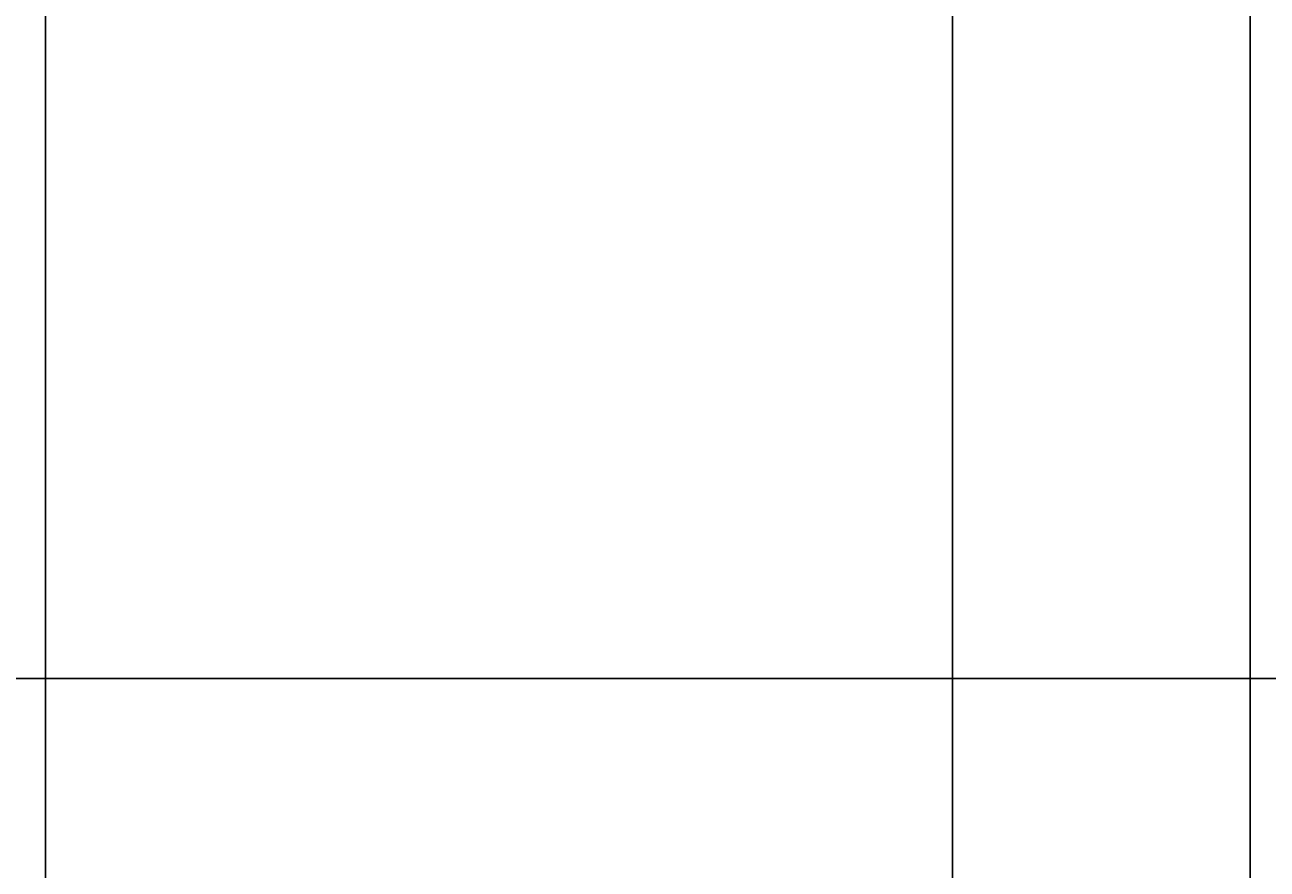
# Model space of a CAD drawing. Units: inches. Extents: x 35362 to 73946, y 43607 to 67532.
# Tile 55 of 134: x 50119 to 51337, y 45263 to 46091. Entities that reach past the tile are written whole.
import ezdxf

# ---------------------------------------------------------------- set-up
doc = ezdxf.new("R2010")
doc.units = ezdxf.units.IN
doc.header["$MEASUREMENT"] = 0
doc.layers.add('A-ANNO-DIMS', color=2, linetype='Continuous', lineweight=18)
doc.styles.get("Standard").update_dxf_attribs({"font": 'arial.ttf'})
doc.dimstyles.get("Standard").update_dxf_attribs({"dimtxt": 0.18, "dimasz": 0.18, "dimexe": 0.18, "dimexo": 0.0625, "dimgap": 0.09, "dimtad": 0, "dimtih": 1, "dimtoh": 1, "dimdec": 4, "dimzin": 0, "dimdsep": 46, "dimtxsty": 'Standard', "dimcen": 0.09, "dimadec": 0, "dimazin": 0, "dimtfac": 1, "dimtdec": 4, "dimtofl": 0, "dimtmove": 0, "dimatfit": 3, "dimfxl": 1, "dimtolj": 1, "dimtzin": 0, "dimarcsym": 0})

# ---------------------------------------------------------------- blocks, each defined once
blk = doc.blocks.new('*D5')
at = {"layer": 'A-ANNO-DIMS', "color": 0, "lineweight": -2, "transparency": 16777216}
for p, q in [((37121.9, 46919.3), (37121.9, 43606.7)), ((69871.5, 45449.8), (69871.5, 43606.7)), ((37122.1, 43606.9), (53496.3, 43606.9)), ((69871.3, 43606.9), (53497.2, 43606.9))]:
    blk.add_line(p, q, dxfattribs=at)
at = {"layer": 'A-ANNO-DIMS', "color": 0, "transparency": 16777216}
for points in [[(37122.1, 43606.9), (37122.1, 43606.8), (37121.9, 43606.9)], [(69871.3, 43606.9), (69871.3, 43606.8), (69871.5, 43606.9)]]:
    blk.add_solid(points, dxfattribs=at)
at = {"layer": 'Defpoints', "color": 0, "transparency": 16777216}
for p in [(37121.9, 46919.4), (69871.5, 45449.9), (69871.5, 43606.9)]:
    blk.add_point(p, dxfattribs=at)
at = {"layer": 'A-ANNO-DIMS', "color": 0, "transparency": 16777216, "insert": (53496.7, 43606.9), "char_height": 0.18, "attachment_point": 5}
blk.add_mtext('\\A1;32750', dxfattribs=at)
blk = doc.blocks.new('*D11')
at = {"layer": 'A-ANNO-DIMS', "color": 0, "lineweight": -2, "transparency": 16777216}
for p, q in [((47978.7, 56028.8), (47978.7, 43606.7)), ((53109.8, 56028.8), (53109.8, 43606.7)), ((47978.8, 43606.9), (50543.9, 43606.9)), ((53109.6, 43606.9), (50544.6, 43606.9))]:
    blk.add_line(p, q, dxfattribs=at)
at = {"layer": 'A-ANNO-DIMS', "color": 0, "transparency": 16777216}
for points in [[(47978.8, 43606.9), (47978.8, 43606.8), (47978.7, 43606.9)], [(53109.6, 43606.9), (53109.6, 43606.8), (53109.8, 43606.9)]]:
    blk.add_solid(points, dxfattribs=at)
at = {"layer": 'Defpoints', "color": 0, "transparency": 16777216}
for p in [(47978.7, 56028.8), (53109.8, 56028.8), (53109.8, 43606.9)]:
    blk.add_point(p, dxfattribs=at)
at = {"layer": 'A-ANNO-DIMS', "color": 0, "transparency": 16777216, "insert": (50544.2, 43606.9), "char_height": 0.18, "attachment_point": 5}
blk.add_mtext('\\A1;5131', dxfattribs=at)
blk = doc.blocks.new('*D13')
at = {"layer": 'A-ANNO-DIMS', "color": 0, "lineweight": -2, "transparency": 16777216}
for p, q in [((48373.5, 51694), (48373.5, 43606.7)), ((51029, 51694), (51029, 43606.7)), ((48373.7, 43606.9), (49700.8, 43606.9)), ((51028.9, 43606.9), (49701.7, 43606.9))]:
    blk.add_line(p, q, dxfattribs=at)
at = {"layer": 'A-ANNO-DIMS', "color": 0, "transparency": 16777216}
for points in [[(48373.7, 43606.9), (48373.7, 43606.8), (48373.5, 43606.9)], [(51028.9, 43606.9), (51028.9, 43606.8), (51029, 43606.9)]]:
    blk.add_solid(points, dxfattribs=at)
at = {"layer": 'Defpoints', "color": 0, "transparency": 16777216}
for p in [(48373.5, 51694.1), (51029, 51694.1), (51029, 43606.9)]:
    blk.add_point(p, dxfattribs=at)
at = {"layer": 'A-ANNO-DIMS', "color": 0, "transparency": 16777216, "insert": (49701.3, 43606.9), "char_height": 0.18, "attachment_point": 5}
blk.add_mtext('\\A1;2655.6', dxfattribs=at)
blk = doc.blocks.new('*D17')
at = {"layer": 'A-ANNO-DIMS', "color": 0, "lineweight": -2, "transparency": 16777216}
for p, q in [((49923.3, 61293.2), (49923.3, 43606.7)), ((51913.9, 61293.2), (51913.9, 43606.7)), ((49923.5, 43606.9), (50918.2, 43606.9)), ((51913.8, 43606.9), (50919.1, 43606.9))]:
    blk.add_line(p, q, dxfattribs=at)
at = {"layer": 'A-ANNO-DIMS', "color": 0, "transparency": 16777216}
for points in [[(49923.5, 43606.9), (49923.5, 43606.8), (49923.3, 43606.9)], [(51913.8, 43606.9), (51913.8, 43606.8), (51913.9, 43606.9)]]:
    blk.add_solid(points, dxfattribs=at)
at = {"layer": 'Defpoints', "color": 0, "transparency": 16777216}
for p in [(49923.3, 61293.3), (51913.9, 61293.3), (51913.9, 43606.9)]:
    blk.add_point(p, dxfattribs=at)
at = {"layer": 'A-ANNO-DIMS', "color": 0, "transparency": 16777216, "insert": (50918.6, 43606.9), "char_height": 0.18, "attachment_point": 5}
blk.add_mtext('\\A1;1990.6', dxfattribs=at)
blk = doc.blocks.new('*D67')
at = {"layer": 'A-ANNO-DIMS', "color": 0, "lineweight": -2, "transparency": 16777216}
for p, q in [((56873.5, 53351.5), (35361.8, 53351.5)), ((35361.9, 53351.3), (35361.9, 49400.9)), ((35361.9, 45450.1), (35361.9, 49400.5)), ((53793.6, 45449.9), (35361.8, 45449.9))]:
    blk.add_line(p, q, dxfattribs=at)
at = {"layer": 'A-ANNO-DIMS', "color": 0, "transparency": 16777216}
for points in [[(35361.9, 53351.3), (35362, 53351.3), (35361.9, 53351.5)], [(35361.9, 45450.1), (35362, 45450.1), (35361.9, 45449.9)]]:
    blk.add_solid(points, dxfattribs=at)
at = {"layer": 'Defpoints', "color": 0, "transparency": 16777216}
for p in [(35361.9, 53351.5), (56873.6, 53351.5), (53793.6, 45449.9)]:
    blk.add_point(p, dxfattribs=at)
at = {"layer": 'A-ANNO-DIMS', "color": 0, "transparency": 16777216, "insert": (35361.9, 49400.7), "char_height": 0.18, "attachment_point": 5}
blk.add_mtext('\\A1;7901.6', dxfattribs=at)
blk = doc.blocks.new('*D107')
at = {"layer": 'A-ANNO-DIMS', "color": 0, "lineweight": -2, "transparency": 16777216}
for p, q in [((50139.6, 59850), (50139.6, 43606.7)), ((51320.8, 59850), (51320.8, 43606.7)), ((50139.7, 43606.9), (50729.7, 43606.9)), ((51320.6, 43606.9), (50730.6, 43606.9))]:
    blk.add_line(p, q, dxfattribs=at)
at = {"layer": 'A-ANNO-DIMS', "color": 0, "transparency": 16777216}
for points in [[(50139.7, 43606.9), (50139.7, 43606.8), (50139.6, 43606.9)], [(51320.6, 43606.9), (51320.6, 43606.8), (51320.8, 43606.9)]]:
    blk.add_solid(points, dxfattribs=at)
at = {"layer": 'Defpoints', "color": 0, "transparency": 16777216}
for p in [(50139.6, 59850.1), (51320.8, 59850.1), (51320.8, 43606.9)]:
    blk.add_point(p, dxfattribs=at)
at = {"layer": 'A-ANNO-DIMS', "color": 0, "transparency": 16777216, "insert": (50730.2, 43606.9), "char_height": 0.18, "attachment_point": 5}
blk.add_mtext('\\A1;1181.3', dxfattribs=at)

msp = doc.modelspace()

# ---------------------------------------------------------------- dimensions: what is measured, and where the dimension line sits
at = {"layer": 'A-ANNO-DIMS'}
for base, p1, p2, override, picture, middle in [((51913.931, 43606.859), (49923.307, 61293.286), (51913.931, 61293.286), {"dimdec": 1, "dimlfac": 1, "dimrnd": 0, "dimzin": 0, "dimdsep": 46, "dimlunit": 2}, '*D17', (50918.619, 43606.859)), ((51320.8133, 43606.859), (50139.5627, 59850.0769), (51320.8133, 59850.0769), {"dimdec": 1, "dimlfac": 1, "dimrnd": 0, "dimzin": 0, "dimdsep": 46, "dimlunit": 2}, '*D107', (50730.188, 43606.859)), ((53109.76, 43606.859), (47978.665, 56028.836), (53109.76, 56028.836), {"dimdec": 0, "dimlfac": 1, "dimrnd": 0, "dimzin": 0, "dimdsep": 46, "dimlunit": 2}, '*D11', (50544.212, 43606.859)), ((51029.043, 43606.859), (48373.492, 51694.087), (51029.043, 51694.087), {"dimdec": 1, "dimlfac": 1, "dimrnd": 0, "dimzin": 0, "dimdsep": 46, "dimlunit": 2}, '*D13', (49701.267, 43606.859)), ((69871.496, 43606.859), (37121.949, 46919.381), (69871.496, 45449.894), {"dimdec": 0, "dimlfac": 1, "dimrnd": 0, "dimzin": 0, "dimdsep": 46, "dimlunit": 2}, '*D5', (53496.723, 43606.859))]:
    dim = msp.add_linear_dim(base=base, p1=p1, p2=p2, dimstyle='Standard', override=override, dxfattribs=at)
    dim.commit()
    dim.dimension.update_dxf_attribs({"geometry": picture, "text_midpoint": middle})
dim = msp.add_linear_dim(base=(35361.949, 53351.529), p1=(53793.638, 45449.894), p2=(56873.602, 53351.529), angle=90, dimstyle='Standard', override={"dimdec": 1, "dimlfac": 1, "dimrnd": 0, "dimzin": 0, "dimdsep": 46, "dimlunit": 2}, dxfattribs=at)
dim.commit()
dim.dimension.update_dxf_attribs({"geometry": '*D67', "text_midpoint": (35361.949, 49400.712)})

doc.saveas('drawing.dxf')
